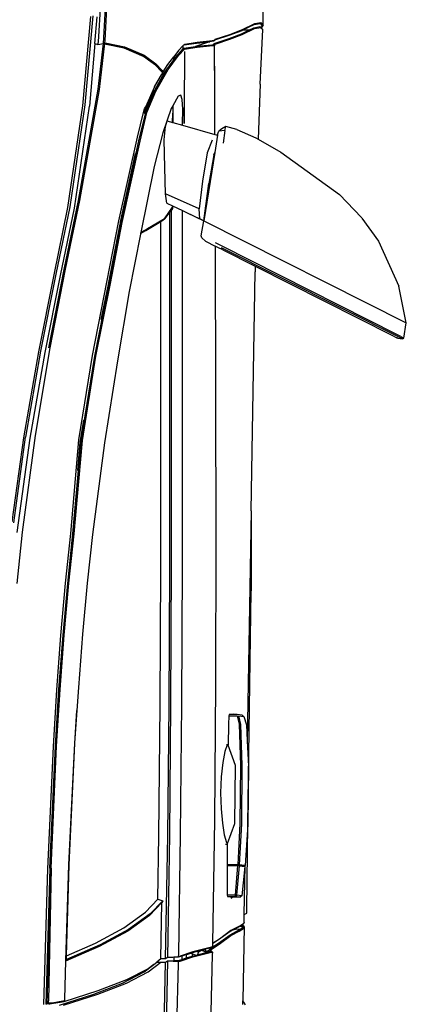
# Model space of a CAD drawing. Units: inches. Extents: x 22042254 to 25404563, y 17568978 to 17626777.
# Tile 31 of 45: x 22179875 to 22179896, y 17626279 to 17626332. Entities that reach past the tile are written whole.
import ezdxf

# ---------------------------------------------------------------- set-up
doc = ezdxf.new("R2010")
doc.units = ezdxf.units.IN
doc.header["$MEASUREMENT"] = 0
doc.layers.add('A-SITE-VEHI', color=8, linetype='Continuous', lineweight=18)
doc.layers.add('Edges', color=250, linetype='Continuous')

# ---------------------------------------------------------------- blocks, each defined once
blk = doc.blocks.new('Nissan Qashqai pl')
at = {"layer": 'Edges'}
for p, q in [((8.8918, 12.7444), (9.0186, 12.9956)), ((9.0386, 12.9907), (8.9254, 12.7664)), ((9.0186, 12.9956), (8.9731, 12.9865)), ((9.0374, 12.9925), (9.0186, 12.9956)), ((9.0356, 12.9888), (9.0333, 12.9845)), ((9.0356, 12.9888), (9.0374, 12.9925)), ((9.0386, 12.9907), (9.0374, 12.9925)), ((9.0376, 12.985), (9.0386, 12.9907)), ((8.9173, 12.961), (8.9731, 12.9865)), ((9.0333, 12.9845), (8.9232, 12.7662)), ((8.9483, 12.8082), (9.0343, 12.9785)), ((9.0343, 12.9785), (9.0347, 12.9794)), ((9.0347, 12.9794), (9.0362, 12.9822)), ((9.0362, 12.9822), (9.037, 12.9838)), ((9.0371, 12.9841), (9.037, 12.9838)), ((9.0371, 12.9841), (9.0376, 12.985)), ((9.0376, 12.985), (9.0371, 12.9847)), ((8.8885, 12.9405), (8.9173, 12.961)), ((8.8591, 12.9127), (8.8879, 12.94)), ((8.8885, 12.9405), (8.8879, 12.94)), ((8.8066, 12.84), (8.8591, 12.9127)), ((8.7908, 12.812), (8.8066, 12.84)), ((8.6489, 12.8179), (8.5719, 12.8193)), ((8.646, 12.8153), (8.6489, 12.8179)), ((8.6489, 12.8179), (8.6527, 12.8156)), ((8.6547, 12.8176), (8.6537, 12.8167)), ((8.7222, 12.8144), (8.6547, 12.8176)), ((8.646, 12.8153), (8.646, 12.8153)), ((8.6472, 12.8076), (8.646, 12.8153)), ((8.647, 12.8142), (8.6498, 12.8168)), ((8.6482, 12.8067), (8.647, 12.8142)), ((8.6546, 12.7926), (8.6472, 12.8076)), ((8.655, 12.7929), (8.6482, 12.8067)), ((8.6498, 12.8168), (8.6524, 12.8153)), ((8.651, 12.814), (8.652, 12.815)), ((8.6524, 12.8064), (8.651, 12.814)), ((8.652, 12.815), (8.6524, 12.8153)), ((8.6534, 12.8073), (8.652, 12.815)), ((8.6524, 12.8153), (8.6527, 12.8156)), ((8.655, 12.801), (8.6524, 12.8064)), ((8.6527, 12.8156), (8.6537, 12.8167)), ((8.6608, 12.7921), (8.6534, 12.8073)), ((8.6537, 12.8167), (8.6537, 12.8166)), ((8.7222, 12.8144), (8.7908, 12.812)), ((8.7785, 12.7855), (8.7891, 12.8089)), ((8.7891, 12.8089), (8.7908, 12.812)), ((8.928, 12.7679), (8.9483, 12.8082)), ((8.9483, 12.8082), (8.9552, 12.8081)), ((9.2517, 12.8031), (8.9552, 12.8081)), ((8.6606, 12.7768), (8.6546, 12.7926)), ((8.6598, 12.7913), (8.655, 12.801)), ((8.655, 12.7929), (8.655, 12.801)), ((8.6556, 12.7918), (8.655, 12.7929)), ((8.655, 12.7922), (8.655, 12.7929)), ((9.2517, 12.8031), (9.351, 12.803)), ((9.2517, 12.8031), (9.5372, 12.7983)), ((9.641, 12.7991), (9.351, 12.803)), ((9.5052, 12.7918), (9.5069, 12.7941)), ((9.5061, 12.7878), (9.5069, 12.7941)), ((9.5069, 12.7941), (9.5176, 12.7972)), ((9.5176, 12.7972), (9.5372, 12.7983)), ((9.5372, 12.7983), (9.5689, 12.7999)), ((9.5689, 12.7999), (9.641, 12.7991)), ((9.641, 12.7991), (9.6921, 12.7956)), ((9.7466, 12.7978), (9.641, 12.7991)), ((9.692, 12.7943), (9.6913, 12.7886)), ((9.6921, 12.7956), (9.692, 12.7943)), ((9.6922, 12.7943), (9.692, 12.7943)), ((9.6922, 12.7943), (9.6921, 12.7956)), ((9.7526, 12.7946), (9.6921, 12.7956)), ((9.6922, 12.7885), (9.693, 12.7955)), ((9.6922, 12.7885), (9.6922, 12.7943)), ((9.693, 12.7955), (9.7296, 12.7914)), ((9.7511, 12.7979), (9.7466, 12.7978)), ((9.7526, 12.7946), (9.7511, 12.7979)), ((9.7623, 12.7945), (9.7526, 12.7946)), ((9.7623, 12.7945), (9.7643, 12.7937)), ((9.7643, 12.7937), (9.7652, 12.7927)), ((9.7643, 12.7937), (9.7648, 12.7929)), ((9.7648, 12.7929), (9.7648, 12.7929)), ((9.7648, 12.7929), (9.7664, 12.7902)), ((9.7652, 12.7927), (9.7665, 12.7907)), ((9.7667, 12.7933), (9.7665, 12.7907)), ((9.7677, 12.7944), (9.7667, 12.7933)), ((9.7676, 12.7931), (9.7667, 12.7933)), ((9.7673, 12.7899), (9.7676, 12.7931)), ((9.769, 12.7926), (9.7676, 12.7931)), ((9.7677, 12.7944), (9.7677, 12.7944)), ((9.77, 12.7936), (9.7677, 12.7944)), ((9.7677, 12.7944), (9.8598, 12.7928)), ((9.7712, 12.7892), (9.769, 12.7926)), ((9.7734, 12.7884), (9.77, 12.7936)), ((9.8598, 12.7928), (9.8614, 12.7937)), ((9.8643, 12.7927), (9.8598, 12.7928)), ((9.8614, 12.7937), (9.8647, 12.7956)), ((8.6616, 12.7758), (8.6556, 12.7918)), ((8.6657, 12.7758), (8.6598, 12.7913)), ((8.6667, 12.7767), (8.6608, 12.7921)), ((8.7785, 12.7855), (8.7751, 12.7719)), ((9.5037, 12.7806), (9.5045, 12.7814)), ((9.5052, 12.7918), (9.5044, 12.7856)), ((9.5044, 12.7856), (9.5045, 12.7814)), ((9.5045, 12.7814), (9.5045, 12.7759)), ((9.5168, 12.7904), (9.5061, 12.7878)), ((9.5061, 12.7856), (9.5167, 12.7883)), ((9.5063, 12.7755), (9.5061, 12.7856)), ((9.5167, 12.7883), (9.5679, 12.7899)), ((9.5679, 12.792), (9.5168, 12.7904)), ((9.5678, 12.7837), (9.5426, 12.7747)), ((9.64, 12.7831), (9.5678, 12.7837)), ((9.6401, 12.7914), (9.5679, 12.792)), ((9.5679, 12.7899), (9.64, 12.7892)), ((9.64, 12.7892), (9.6912, 12.7865)), ((9.6645, 12.7737), (9.64, 12.7831)), ((9.6913, 12.7886), (9.6401, 12.7914)), ((9.6912, 12.7811), (9.6911, 12.7796)), ((9.6913, 12.7886), (9.6912, 12.7865)), ((9.6912, 12.7865), (9.6912, 12.7811)), ((9.692, 12.7811), (9.6912, 12.7811)), ((9.692, 12.7811), (9.6921, 12.7864)), ((9.692, 12.7796), (9.692, 12.7811)), ((9.6922, 12.7885), (9.6921, 12.7864)), ((9.6921, 12.7864), (9.7288, 12.7832)), ((9.7288, 12.7854), (9.6922, 12.7885)), ((9.7288, 12.7832), (9.7287, 12.7734)), ((9.7296, 12.7914), (9.7288, 12.7854)), ((9.7306, 12.7834), (9.7288, 12.7854)), ((9.7288, 12.7854), (9.7288, 12.7832)), ((9.7288, 12.7832), (9.7306, 12.7834)), ((9.7296, 12.7914), (9.7314, 12.7895)), ((9.7305, 12.7738), (9.7306, 12.7834)), ((9.7306, 12.7834), (9.7314, 12.7895)), ((9.7314, 12.7895), (9.7313, 12.7798)), ((9.7665, 12.7904), (9.7664, 12.7902)), ((9.7664, 12.7902), (9.7674, 12.7885)), ((9.7665, 12.7907), (9.7676, 12.7889)), ((9.7673, 12.7897), (9.7673, 12.7899)), ((9.7673, 12.7897), (9.7676, 12.7889)), ((9.7674, 12.7885), (9.7728, 12.7781)), ((9.7676, 12.7889), (9.7684, 12.7875)), ((9.7676, 12.7887), (9.7678, 12.7882)), ((9.7684, 12.7875), (9.7717, 12.781)), ((9.7707, 12.7848), (9.7709, 12.7893)), ((9.7717, 12.781), (9.7707, 12.7848)), ((9.7709, 12.7893), (9.7712, 12.7892)), ((9.7724, 12.7874), (9.7712, 12.7892)), ((9.7717, 12.781), (9.7738, 12.7771)), ((9.7778, 12.777), (9.7724, 12.7874)), ((9.7788, 12.778), (9.7734, 12.7884)), ((8.6667, 12.7584), (8.6606, 12.7768)), ((8.6675, 12.758), (8.6616, 12.7758)), ((8.6718, 12.7574), (8.6657, 12.7758)), ((8.6728, 12.7584), (8.6667, 12.7767)), ((8.7751, 12.7719), (8.7779, 12.7668)), ((8.7798, 12.7703), (8.7751, 12.7719)), ((8.7798, 12.7703), (8.7807, 12.763)), ((8.7798, 12.7703), (8.7954, 12.7683)), ((9.5045, 12.7759), (9.5063, 12.7755)), ((9.5063, 12.7755), (9.5168, 12.7751)), ((9.5168, 12.7751), (9.5423, 12.7746)), ((9.5423, 12.7746), (9.5422, 12.7736)), ((9.5422, 12.7736), (9.5422, 12.7725)), ((9.5422, 12.7736), (9.5424, 12.7735)), ((9.5426, 12.7747), (9.5423, 12.7746)), ((9.5426, 12.7747), (9.5424, 12.7735)), ((9.5424, 12.7735), (9.5503, 12.7706)), ((9.5503, 12.7706), (9.5641, 12.7681)), ((9.6395, 12.7676), (9.654, 12.7697)), ((9.654, 12.7697), (9.6633, 12.7726)), ((9.6633, 12.7726), (9.6645, 12.7737)), ((9.6655, 12.7733), (9.6645, 12.7737)), ((9.6655, 12.7733), (9.6911, 12.7732)), ((9.6655, 12.7713), (9.6655, 12.7733)), ((9.6911, 12.7796), (9.6911, 12.7732)), ((9.6911, 12.7732), (9.692, 12.7733)), ((9.692, 12.7733), (9.692, 12.7796)), ((9.692, 12.7733), (9.7287, 12.7734)), ((9.7287, 12.7734), (9.7305, 12.7738)), ((9.7305, 12.7738), (9.7313, 12.7798)), ((9.733, 12.7782), (9.7313, 12.7798)), ((9.7728, 12.7781), (9.7832, 12.7637)), ((9.7738, 12.7771), (9.7842, 12.7627)), ((9.7883, 12.7626), (9.7778, 12.777)), ((9.7894, 12.7636), (9.7788, 12.778)), ((8.6675, 12.758), (8.6667, 12.7584)), ((8.6679, 12.7578), (8.6675, 12.758)), ((8.6676, 12.7576), (8.6675, 12.7576)), ((8.6675, 12.7576), (8.6675, 12.7576)), ((8.6675, 12.7576), (8.6676, 12.7576)), ((8.6676, 12.7576), (8.6677, 12.7576)), ((8.6677, 12.7576), (8.6677, 12.7576)), ((8.6677, 12.7576), (8.6682, 12.7576)), ((8.6682, 12.7576), (8.6679, 12.7578)), ((8.6682, 12.7576), (8.6692, 12.7566)), ((8.6682, 12.7572), (8.6682, 12.7576)), ((8.6684, 12.7554), (8.6682, 12.7572)), ((8.6682, 12.7572), (8.6692, 12.7566)), ((8.6692, 12.7566), (8.6697, 12.7519)), ((8.6729, 12.7568), (8.6718, 12.7574)), ((8.674, 12.7578), (8.6728, 12.7584)), ((8.6733, 12.7566), (8.6729, 12.7568)), ((8.6735, 12.7544), (8.6733, 12.7566)), ((8.6742, 12.7576), (8.674, 12.7578)), ((8.6742, 12.7584), (8.6743, 12.7582)), ((8.6744, 12.755), (8.6742, 12.7576)), ((8.6744, 12.7576), (8.6742, 12.7576)), ((8.6744, 12.7578), (8.6744, 12.7576)), ((8.6773, 12.7577), (8.6744, 12.7576)), ((8.6791, 12.7578), (8.677, 12.7578)), ((8.6791, 12.7577), (8.6773, 12.7577)), ((8.7205, 12.7579), (8.6791, 12.7578)), ((8.6791, 12.7577), (8.6791, 12.7578)), ((8.6878, 12.7577), (8.6791, 12.7578)), ((8.6878, 12.7577), (8.6791, 12.7577)), ((8.6878, 12.7577), (8.6878, 12.7577)), ((8.6911, 12.7577), (8.6878, 12.7577)), ((8.7205, 12.7579), (8.6911, 12.7577)), ((8.7849, 12.7582), (8.7205, 12.7579)), ((8.7734, 12.7181), (8.7849, 12.7582)), ((8.7779, 12.7668), (8.7807, 12.763)), ((8.7849, 12.7615), (8.7807, 12.763)), ((8.7849, 12.7615), (8.7858, 12.7613)), ((8.7849, 12.7582), (8.7856, 12.7608)), ((8.7858, 12.7613), (8.7856, 12.7608)), ((8.7858, 12.7613), (8.807, 12.758)), ((8.8102, 12.7568), (8.807, 12.758)), ((8.807, 12.758), (8.8918, 12.7444)), ((8.8102, 12.7568), (8.8455, 12.7506)), ((8.9171, 12.7464), (8.9233, 12.7586)), ((8.9232, 12.7662), (8.9194, 12.7588)), ((8.925, 12.762), (8.9233, 12.7586)), ((8.9233, 12.7586), (9.2886, 12.7594)), ((8.928, 12.7679), (8.925, 12.762)), ((9.2886, 12.7594), (9.4673, 12.7589)), ((9.4673, 12.7589), (9.6358, 12.7575)), ((9.5641, 12.7681), (9.5818, 12.766)), ((9.5818, 12.766), (9.6016, 12.7651)), ((9.6016, 12.7651), (9.6215, 12.766)), ((9.6215, 12.766), (9.6395, 12.7676)), ((9.6358, 12.7575), (9.7887, 12.7552)), ((9.7832, 12.7637), (9.7887, 12.7552)), ((9.7842, 12.7627), (9.7891, 12.7552)), ((9.7933, 12.7549), (9.7883, 12.7626)), ((9.7965, 12.7526), (9.7894, 12.7636)), ((8.6684, 12.7554), (8.6685, 12.7549)), ((8.6684, 12.755), (8.6684, 12.7554)), ((8.6703, 12.7361), (8.6684, 12.755)), ((8.6697, 12.7519), (8.6698, 12.7516)), ((8.6714, 12.7353), (8.6697, 12.7519)), ((8.6698, 12.7516), (8.6755, 12.7343)), ((8.6754, 12.7353), (8.6735, 12.7544)), ((8.6764, 12.736), (8.6744, 12.755)), ((8.7917, 12.7547), (8.8075, 12.7486)), ((8.8075, 12.7486), (8.8429, 12.7426)), ((8.8918, 12.7444), (8.8455, 12.7506)), ((8.8815, 12.7228), (8.892, 12.7444)), ((8.892, 12.7444), (8.8908, 12.7421)), ((8.8911, 12.7428), (8.8919, 12.7444)), ((8.8911, 12.7428), (8.8919, 12.7444)), ((8.8919, 12.7444), (8.8911, 12.7428)), ((8.8919, 12.7444), (8.8918, 12.7444)), ((8.892, 12.7444), (8.8919, 12.7444)), ((8.8919, 12.7444), (8.8919, 12.7444)), ((8.8919, 12.7444), (8.8919, 12.7444)), ((8.9106, 12.7413), (8.892, 12.7444)), ((8.892, 12.7444), (8.892, 12.7444)), ((8.9171, 12.7464), (8.9131, 12.7421)), ((8.9171, 12.7464), (8.917, 12.7468)), ((9.7887, 12.7552), (9.7891, 12.7552)), ((9.7891, 12.7552), (9.79, 12.7552)), ((9.79, 12.7552), (9.7931, 12.7552)), ((9.7931, 12.7552), (9.7934, 12.7535)), ((9.7931, 12.7552), (9.7933, 12.7549)), ((9.7933, 12.7549), (9.7941, 12.7541)), ((9.7934, 12.7535), (9.7938, 12.7538)), ((9.7934, 12.7535), (9.7937, 12.7524)), ((9.7937, 12.7524), (9.7992, 12.7308)), ((9.7941, 12.7541), (9.7943, 12.7535)), ((9.7955, 12.7516), (9.7943, 12.7535)), ((9.7943, 12.7535), (9.7964, 12.7453)), ((9.7963, 12.7523), (9.7955, 12.7516)), ((9.7963, 12.7523), (9.7963, 12.7524)), ((9.7964, 12.7524), (9.7963, 12.7523)), ((9.7992, 12.7476), (9.7963, 12.7523)), ((9.7967, 12.7526), (9.7964, 12.7524)), ((9.7964, 12.7525), (9.7964, 12.7524)), ((9.7964, 12.7524), (9.7996, 12.7475)), ((9.7964, 12.7453), (9.7992, 12.7476)), ((9.7964, 12.7453), (9.7973, 12.7418)), ((9.7983, 12.7541), (9.7965, 12.7526)), ((9.7965, 12.7526), (9.7967, 12.7526)), ((9.7977, 12.7535), (9.7967, 12.7526)), ((9.7967, 12.7526), (9.7986, 12.7526)), ((9.7982, 12.754), (9.7977, 12.7535)), ((9.7977, 12.7444), (9.7985, 12.7451)), ((9.7985, 12.7451), (9.7977, 12.7431)), ((9.7977, 12.7431), (9.7977, 12.7444)), ((9.7983, 12.7541), (9.7982, 12.754)), ((9.7986, 12.7526), (9.7982, 12.754)), ((9.7986, 12.7544), (9.7983, 12.7541)), ((9.7989, 12.7461), (9.7985, 12.7451)), ((9.7993, 12.755), (9.7986, 12.7544)), ((9.7988, 12.7516), (9.7986, 12.7526)), ((9.7998, 12.7477), (9.7988, 12.7516)), ((9.7998, 12.7466), (9.7989, 12.7461)), ((9.7998, 12.7466), (9.7992, 12.7476)), ((9.7999, 12.7522), (9.7993, 12.755)), ((9.7993, 12.755), (9.8024, 12.7549)), ((9.7996, 12.7475), (9.7998, 12.7477)), ((9.8002, 12.7461), (9.7996, 12.7475)), ((9.8001, 12.7468), (9.7996, 12.7475)), ((9.8001, 12.7468), (9.7998, 12.7477)), ((9.8003, 12.7458), (9.7998, 12.7466)), ((9.8054, 12.7307), (9.7999, 12.7522)), ((9.8002, 12.7461), (9.8001, 12.7468)), ((9.8003, 12.7458), (9.8002, 12.7461)), ((9.8027, 12.7364), (9.8003, 12.7458)), ((9.8024, 12.7549), (9.9426, 12.7518)), ((8.6727, 12.7207), (8.6703, 12.7361)), ((8.6737, 12.7197), (8.6714, 12.7353)), ((8.6755, 12.7343), (8.6754, 12.7353)), ((8.6777, 12.7196), (8.6755, 12.7343)), ((8.6764, 12.7359), (8.6764, 12.736)), ((8.6788, 12.7205), (8.6764, 12.7359)), ((8.8429, 12.7426), (8.8771, 12.7388)), ((8.8771, 12.7388), (8.8585, 12.6969)), ((8.8895, 12.7393), (8.8771, 12.7388)), ((8.8815, 12.7228), (8.8895, 12.7393)), ((8.8908, 12.7421), (8.8895, 12.7393)), ((8.8906, 12.7418), (8.8895, 12.7393)), ((8.8906, 12.7418), (8.8911, 12.7428)), ((8.9131, 12.7421), (8.9106, 12.7413)), ((9.7977, 12.7431), (9.7973, 12.7418)), ((9.7973, 12.7418), (9.7977, 12.7409)), ((9.7973, 12.7418), (9.7977, 12.7399)), ((9.7977, 12.7399), (9.7977, 12.7409)), ((9.7977, 12.7409), (9.7987, 12.7388)), ((9.7977, 12.7399), (9.7978, 12.7397)), ((9.7987, 12.7388), (9.7978, 12.7397)), ((9.7978, 12.7397), (9.7987, 12.7362)), ((9.7987, 12.7388), (9.7992, 12.7377)), ((9.7987, 12.7362), (9.7992, 12.7377)), ((9.7987, 12.7362), (9.8002, 12.7301)), ((9.7992, 12.7377), (9.8027, 12.7364)), ((9.8014, 12.7303), (9.8031, 12.7349)), ((9.8031, 12.7349), (9.8027, 12.7364)), ((9.8043, 12.7303), (9.8031, 12.7349)), ((8.6737, 12.7197), (8.6727, 12.7207)), ((8.6746, 12.7189), (8.6737, 12.7197)), ((8.6785, 12.7189), (8.6777, 12.7196)), ((8.687, 12.7132), (8.6788, 12.7205)), ((8.6818, 12.7204), (8.7012, 12.7203)), ((8.7012, 12.7203), (8.7012, 12.7203)), ((8.7012, 12.7203), (8.7026, 12.7203)), ((8.7026, 12.7203), (8.7026, 12.7203)), ((8.7026, 12.7203), (8.7072, 12.7203)), ((8.7072, 12.7203), (8.7072, 12.7203)), ((8.7072, 12.7203), (8.7273, 12.7202)), ((8.7273, 12.7202), (8.7273, 12.7201)), ((8.7273, 12.7202), (8.7354, 12.7202)), ((8.7354, 12.7201), (8.7354, 12.7202)), ((8.7354, 12.7202), (8.742, 12.7202)), ((8.742, 12.7201), (8.742, 12.7202)), ((8.742, 12.7202), (8.742, 12.7201)), ((8.742, 12.7202), (8.742, 12.7202)), ((8.742, 12.7202), (8.7426, 12.7202)), ((8.7426, 12.7201), (8.7426, 12.7202)), ((8.7426, 12.7202), (8.7433, 12.7202)), ((8.7433, 12.7201), (8.7433, 12.7202)), ((8.7433, 12.7202), (8.7711, 12.7201)), ((8.7711, 12.7201), (8.7516, 12.72)), ((8.8793, 12.7181), (8.8815, 12.7228)), ((9.7992, 12.7308), (9.8044, 12.7151)), ((9.8002, 12.7301), (9.8008, 12.7285)), ((9.8008, 12.7285), (9.8014, 12.7303)), ((9.8008, 12.7285), (9.8014, 12.7265)), ((9.8043, 12.7303), (9.8014, 12.7303)), ((9.8014, 12.7265), (9.803, 12.723)), ((9.8014, 12.7265), (9.8026, 12.723)), ((9.803, 12.723), (9.8026, 12.723)), ((9.8026, 12.723), (9.8046, 12.7171)), ((9.8067, 12.7229), (9.803, 12.723)), ((9.8044, 12.73), (9.8043, 12.7303)), ((9.8067, 12.7229), (9.8044, 12.73)), ((9.8106, 12.715), (9.8054, 12.7307)), ((9.8086, 12.7171), (9.8067, 12.7229)), ((8.6785, 12.7189), (8.6746, 12.7189)), ((8.6805, 12.7132), (8.6746, 12.7189)), ((8.6815, 12.7162), (8.6785, 12.7189)), ((8.6805, 12.7132), (8.6884, 12.7071)), ((8.6815, 12.7162), (8.6818, 12.7154)), ((8.6817, 12.716), (8.6815, 12.7162)), ((8.6817, 12.716), (8.6818, 12.7154)), ((8.6859, 12.7122), (8.6817, 12.716)), ((8.6818, 12.7154), (8.6902, 12.7081)), ((8.6927, 12.7071), (8.6859, 12.7122)), ((8.7042, 12.7002), (8.687, 12.7132)), ((8.6917, 12.7071), (8.6884, 12.7071)), ((8.698, 12.6996), (8.6884, 12.7071)), ((8.6902, 12.7081), (8.6917, 12.7071)), ((8.6917, 12.7071), (8.7075, 12.6955)), ((8.6927, 12.7071), (8.6923, 12.7071)), ((8.7032, 12.6992), (8.6927, 12.7071)), ((8.7415, 12.7177), (8.7361, 12.7158)), ((8.7361, 12.7158), (8.7373, 12.7128)), ((8.7373, 12.7128), (8.7492, 12.7059)), ((8.7534, 12.7185), (8.7415, 12.7177)), ((8.7718, 12.7181), (8.7534, 12.7185)), ((8.7698, 12.7058), (8.7734, 12.7181)), ((8.7734, 12.7181), (8.7718, 12.7181)), ((8.8734, 12.7057), (8.8793, 12.7181)), ((9.3194, 12.7179), (8.8793, 12.7181)), ((9.4919, 12.7173), (9.3194, 12.7179)), ((9.6538, 12.7157), (9.4919, 12.7173)), ((9.802, 12.7133), (9.6538, 12.7157)), ((9.8051, 12.7132), (9.802, 12.7133)), ((9.8044, 12.7151), (9.8051, 12.7132)), ((9.8046, 12.7171), (9.8086, 12.7171)), ((9.8046, 12.7171), (9.8055, 12.7143)), ((9.8061, 12.6994), (9.8051, 12.7132)), ((9.8055, 12.7143), (9.8058, 12.7073)), ((9.8058, 12.7073), (9.8098, 12.7073)), ((9.8058, 12.7073), (9.8061, 12.6994)), ((9.8096, 12.7142), (9.8086, 12.7171)), ((9.8098, 12.7073), (9.8096, 12.7142)), ((9.8101, 12.6993), (9.8098, 12.7073)), ((9.8101, 12.6993), (9.8112, 12.7131)), ((9.8112, 12.7131), (9.8106, 12.715)), ((9.8143, 12.713), (9.8112, 12.7131)), ((9.9414, 12.71), (9.8143, 12.713)), ((8.7071, 12.6942), (8.698, 12.6996)), ((8.7302, 12.684), (8.7032, 12.6992)), ((8.7312, 12.6851), (8.7042, 12.7002)), ((8.7075, 12.6955), (8.7346, 12.6806)), ((8.7492, 12.7059), (8.7572, 12.7062)), ((8.7492, 12.7059), (8.7524, 12.704)), ((8.7524, 12.704), (8.7828, 12.6934)), ((8.7572, 12.7062), (8.7698, 12.7058)), ((8.7698, 12.7057), (8.7583, 12.706)), ((8.7678, 12.6988), (8.7698, 12.7057)), ((8.7748, 12.6967), (8.7678, 12.6988)), ((8.7698, 12.7057), (8.7698, 12.7058)), ((8.7916, 12.6954), (8.7748, 12.6967)), ((8.8259, 12.6959), (8.7916, 12.6954)), ((8.8585, 12.6969), (8.8259, 12.6959)), ((8.87, 12.6987), (8.8585, 12.6969)), ((8.87, 12.6987), (8.8734, 12.7057)), ((8.8734, 12.7057), (8.8768, 12.7057)), ((8.8751, 12.7054), (8.8768, 12.7057)), ((8.8893, 12.6956), (8.8751, 12.7054)), ((8.8768, 12.7057), (8.879, 12.704)), ((8.879, 12.704), (9.3198, 12.7039)), ((8.879, 12.704), (8.881, 12.7023)), ((9.3225, 12.7021), (8.881, 12.7023)), ((8.881, 12.7023), (8.8893, 12.6956)), ((8.8893, 12.6956), (8.9021, 12.6745)), ((8.8913, 12.6936), (8.8893, 12.6956)), ((9.3198, 12.7039), (9.4922, 12.7033)), ((9.4936, 12.7013), (9.3225, 12.7021)), ((9.4922, 12.7033), (9.654, 12.7018)), ((9.6552, 12.6997), (9.4936, 12.7013)), ((9.654, 12.7018), (9.8061, 12.6994)), ((9.8078, 12.6971), (9.6552, 12.6997)), ((9.8061, 12.6994), (9.8078, 12.6971)), ((9.8078, 12.6971), (9.8078, 12.6913)), ((9.8119, 12.697), (9.8101, 12.6993)), ((9.8101, 12.6993), (9.9411, 12.6966)), ((9.9393, 12.6944), (9.8119, 12.697)), ((9.8119, 12.6912), (9.8119, 12.697)), ((8.6864, 12.6706), (8.697, 12.685)), ((8.6875, 12.6698), (8.6979, 12.6839)), ((8.6987, 12.6845), (8.6924, 12.676)), ((8.697, 12.685), (8.7055, 12.6927)), ((8.6979, 12.6839), (8.7062, 12.6915)), ((8.7062, 12.6915), (8.6987, 12.6845)), ((8.7055, 12.6927), (8.7071, 12.6942)), ((8.7062, 12.6915), (8.7067, 12.6919)), ((8.7067, 12.6919), (8.7083, 12.6934)), ((8.7071, 12.6942), (8.7083, 12.6934)), ((8.7083, 12.6934), (8.7083, 12.6934)), ((8.7083, 12.6934), (8.7083, 12.6934)), ((8.7102, 12.6923), (8.7083, 12.6934)), ((8.7083, 12.6934), (8.7083, 12.6934)), ((8.7108, 12.6919), (8.7102, 12.6923)), ((8.7102, 12.6923), (8.7102, 12.6923)), ((8.7257, 12.6833), (8.7108, 12.6919)), ((8.7248, 12.6836), (8.7108, 12.6919)), ((8.7257, 12.6833), (8.7248, 12.6836)), ((8.7257, 12.6832), (8.7257, 12.6833)), ((8.7257, 12.6832), (8.7508, 12.672)), ((8.7529, 12.6741), (8.7302, 12.684)), ((8.7574, 12.6737), (8.7312, 12.6851)), ((8.7828, 12.6934), (8.8245, 12.6828)), ((8.8245, 12.6828), (8.9063, 12.6663)), ((8.8927, 12.6913), (8.8913, 12.6936)), ((9.3224, 12.6911), (8.8927, 12.6913)), ((8.9041, 12.6725), (8.8927, 12.6913)), ((9.3225, 12.6911), (9.3224, 12.6911)), ((9.4936, 12.6904), (9.3225, 12.6911)), ((9.6552, 12.6888), (9.4936, 12.6904)), ((9.7337, 12.6875), (9.6552, 12.6888)), ((9.7337, 12.6875), (9.7357, 12.6935)), ((9.7499, 12.6721), (9.7337, 12.6875)), ((9.7357, 12.6935), (9.7378, 12.6924)), ((9.7357, 12.6935), (9.7519, 12.678)), ((9.7378, 12.6924), (9.754, 12.677)), ((9.8078, 12.6913), (9.7378, 12.6924)), ((9.8078, 12.6913), (9.8119, 12.6862)), ((9.8241, 12.6756), (9.8119, 12.6912)), ((9.8119, 12.6862), (9.8119, 12.6912)), ((9.8147, 12.6826), (9.8119, 12.6862)), ((8.6759, 12.6459), (8.6864, 12.6706)), ((8.6883, 12.6704), (8.6777, 12.6457)), ((8.6924, 12.676), (8.6883, 12.6704)), ((8.6924, 12.676), (8.6924, 12.6762)), ((8.7346, 12.6806), (8.7491, 12.6738)), ((8.7346, 12.6806), (8.7577, 12.6709)), ((8.7508, 12.672), (8.7491, 12.6738)), ((8.7491, 12.6738), (8.7576, 12.6699)), ((8.7532, 12.6708), (8.7508, 12.672)), ((8.7529, 12.6741), (8.7577, 12.6709)), ((8.757, 12.6724), (8.7529, 12.6741)), ((8.7575, 12.6698), (8.7532, 12.6708)), ((8.7587, 12.672), (8.757, 12.6724)), ((8.7931, 12.6653), (8.7574, 12.6737)), ((8.7582, 12.6707), (8.7576, 12.6699)), ((8.7577, 12.6709), (8.7582, 12.6707)), ((8.759, 12.6717), (8.7582, 12.6707)), ((8.7587, 12.672), (8.759, 12.6717)), ((8.7591, 12.6719), (8.7587, 12.672)), ((8.7591, 12.6719), (8.759, 12.6717)), ((8.7925, 12.664), (8.7591, 12.6719)), ((8.9021, 12.6745), (8.9063, 12.6663)), ((8.9075, 12.6661), (8.9041, 12.6725)), ((9.7692, 12.6453), (9.7499, 12.6721)), ((9.7519, 12.678), (9.7713, 12.6512)), ((9.754, 12.677), (9.7733, 12.6502)), ((9.8147, 12.6826), (9.8147, 12.6826)), ((9.8147, 12.6826), (9.8201, 12.6756)), ((9.8241, 12.6706), (9.8147, 12.6826)), ((9.8201, 12.6756), (9.8338, 12.6486)), ((9.8378, 12.6485), (9.8241, 12.6756)), ((9.8378, 12.6435), (9.8241, 12.6706)), ((8.6772, 12.6454), (8.6875, 12.6698)), ((8.7576, 12.6699), (8.7575, 12.6698)), ((8.7881, 12.6621), (8.7575, 12.6698)), ((8.8918, 12.6392), (8.7881, 12.6621)), ((8.8941, 12.6418), (8.7925, 12.664)), ((8.8942, 12.6432), (8.7931, 12.6653)), ((8.8083, 12.6591), (8.8954, 12.6403)), ((8.9063, 12.6663), (8.9075, 12.6661)), ((8.9075, 12.6661), (8.9087, 12.6658)), ((8.9087, 12.6658), (8.9797, 12.6518)), ((8.9797, 12.6518), (9.0656, 12.6372)), ((9.7713, 12.6512), (9.7905, 12.6158)), ((9.7733, 12.6502), (9.7925, 12.6148)), ((9.8338, 12.6486), (9.8475, 12.613)), ((9.8516, 12.6129), (9.8378, 12.6485)), ((8.6716, 12.6242), (8.6759, 12.6459)), ((8.6772, 12.6454), (8.6721, 12.6201)), ((8.6777, 12.6457), (8.6727, 12.6213)), ((8.9679, 12.6241), (8.8918, 12.6392)), ((9.0601, 12.6092), (8.8941, 12.6418)), ((8.9696, 12.6285), (8.8942, 12.6432)), ((8.8961, 12.6401), (8.9704, 12.6257)), ((9.0656, 12.6372), (9.1676, 12.6212)), ((9.7885, 12.6099), (9.7692, 12.6453)), ((9.8516, 12.6079), (9.8378, 12.6435)), ((8.6197, 12.6241), (8.6683, 12.6215)), ((8.6721, 12.6201), (8.6204, 12.6229)), ((8.6683, 12.6215), (8.671, 12.6214)), ((8.671, 12.6214), (8.6716, 12.6242)), ((9.0591, 12.6065), (8.9679, 12.6241)), ((9.06, 12.6106), (8.9696, 12.6285)), ((8.9704, 12.6257), (8.9708, 12.6256)), ((8.9708, 12.6256), (9.0143, 12.6169)), ((8.622, 12.6161), (8.6699, 12.6132)), ((8.6721, 12.6093), (8.6387, 12.6123)), ((8.6699, 12.6132), (8.6721, 12.613)), ((8.671, 12.6214), (8.6721, 12.6201)), ((8.6727, 12.6213), (8.6721, 12.6201)), ((8.6733, 12.6129), (8.6721, 12.6201)), ((8.7287, 12.6134), (8.6721, 12.6201)), ((8.6721, 12.6127), (8.6721, 12.613)), ((8.6721, 12.613), (8.6733, 12.6129)), ((8.6721, 12.6093), (8.6733, 12.6129)), ((8.6721, 12.6093), (8.7496, 12.6025)), ((8.6727, 12.6213), (8.6753, 12.621)), ((8.6753, 12.621), (8.7292, 12.6146)), ((8.8666, 12.5888), (8.7287, 12.6134)), ((8.7292, 12.6146), (8.8666, 12.5901)), ((9.1644, 12.5938), (9.06, 12.6106)), ((9.1676, 12.6212), (9.2814, 12.6065)), ((9.8039, 12.5741), (9.7885, 12.6099)), ((9.7905, 12.6158), (9.8087, 12.574)), ((9.7925, 12.6148), (9.8107, 12.573)), ((9.8475, 12.613), (9.8611, 12.5708)), ((9.8652, 12.5704), (9.8516, 12.6129)), ((8.6375, 12.6066), (8.7481, 12.5968)), ((8.6386, 12.6037), (8.7491, 12.594)), ((8.8761, 12.5839), (8.7496, 12.6025)), ((9.1639, 12.5895), (9.0591, 12.6065)), ((9.1645, 12.5924), (9.0601, 12.6092)), ((9.2814, 12.6065), (9.3416, 12.5999)), ((9.3416, 12.5999), (9.4048, 12.5941)), ((9.8652, 12.5654), (9.8516, 12.6079)), ((8.7481, 12.5968), (8.8745, 12.5782)), ((8.7491, 12.594), (8.8754, 12.5755)), ((8.8666, 12.5901), (8.9521, 12.5726)), ((8.9522, 12.5713), (8.8666, 12.5888)), ((9.1393, 12.5951), (9.1647, 12.591)), ((9.2801, 12.5794), (9.1639, 12.5895)), ((9.2803, 12.5836), (9.1644, 12.5938)), ((9.2804, 12.5821), (9.1645, 12.5924)), ((9.1647, 12.591), (9.1668, 12.5908)), ((9.1668, 12.5908), (9.2019, 12.5877)), ((9.4048, 12.5941), (9.471, 12.5888)), ((9.471, 12.5888), (9.4997, 12.5869)), ((9.5404, 12.5844), (9.4997, 12.5869)), ((9.4997, 12.5869), (9.5403, 12.5842)), ((8.8745, 12.5782), (8.9583, 12.5609)), ((8.8754, 12.5755), (8.9591, 12.5583)), ((8.9598, 12.5666), (8.8761, 12.5839)), ((9.3418, 12.5729), (9.2801, 12.5794)), ((9.3418, 12.5771), (9.2803, 12.5836)), ((9.3419, 12.5756), (9.2804, 12.5821)), ((9.4062, 12.5713), (9.3418, 12.5771)), ((9.4064, 12.5671), (9.3418, 12.5729)), ((9.4063, 12.5699), (9.3419, 12.5756)), ((9.5403, 12.5842), (9.6913, 12.5767)), ((9.6912, 12.5774), (9.5404, 12.5844)), ((9.8039, 12.5741), (9.6912, 12.5774)), ((9.6913, 12.5767), (9.8099, 12.573)), ((9.8087, 12.574), (9.8039, 12.5741)), ((9.8099, 12.573), (9.8087, 12.574)), ((9.8099, 12.573), (9.8107, 12.573)), ((9.8107, 12.573), (9.8573, 12.5716)), ((8.9521, 12.5726), (9.0495, 12.5536)), ((9.0497, 12.5523), (8.9522, 12.5713)), ((8.9583, 12.5609), (9.0538, 12.5419)), ((9.0552, 12.5477), (8.9598, 12.5666)), ((9.4735, 12.5663), (9.4062, 12.5713)), ((9.4736, 12.5648), (9.4063, 12.5699)), ((9.4739, 12.5621), (9.4064, 12.5671)), ((9.5437, 12.5619), (9.4735, 12.5663)), ((9.5438, 12.5605), (9.4736, 12.5648)), ((9.5443, 12.5579), (9.4739, 12.5621)), ((9.6953, 12.5549), (9.5437, 12.5619)), ((9.6954, 12.5535), (9.5438, 12.5605)), ((9.8573, 12.5716), (9.8603, 12.5715)), ((9.8603, 12.5715), (9.8605, 12.5696)), ((9.8611, 12.5708), (9.8603, 12.5715)), ((9.8605, 12.5696), (9.8626, 12.5564)), ((9.8612, 12.5707), (9.8611, 12.5708)), ((9.8612, 12.5707), (9.8615, 12.5688)), ((9.8615, 12.5688), (9.8635, 12.5556)), ((8.9591, 12.5583), (9.0546, 12.5394)), ((9.0495, 12.5536), (9.1584, 12.5351)), ((9.696, 12.551), (9.5443, 12.5579)), ((9.6953, 12.5549), (9.8598, 12.5517)), ((9.6953, 12.5549), (9.863, 12.5497)), ((9.6954, 12.5535), (9.8641, 12.5483)), ((9.8644, 12.5459), (9.696, 12.551)), ((9.8629, 12.5516), (9.8598, 12.5517)), ((9.8626, 12.5564), (9.8627, 12.5532)), ((9.8637, 12.5532), (9.8627, 12.5532)), ((9.8627, 12.5532), (9.8629, 12.5516)), ((9.8629, 12.5516), (9.863, 12.5497)), ((9.8641, 12.5483), (9.863, 12.5497)), ((9.8635, 12.5556), (9.8637, 12.5532)), ((9.8643, 12.5532), (9.8637, 12.5532)), ((9.8637, 12.5532), (9.8638, 12.5508)), ((9.8638, 12.5508), (9.8641, 12.5483)), ((9.0538, 12.5419), (9.1605, 12.5233)), ((9.0546, 12.5394), (9.1612, 12.5208)), ((9.1617, 12.5292), (9.0552, 12.5477)), ((9.1584, 12.5351), (9.2783, 12.5191)), ((9.2789, 12.5131), (9.1617, 12.5292)), ((9.2669, 12.5088), (9.1605, 12.5233)), ((9.1612, 12.5208), (9.2656, 12.5065)), ((9.2783, 12.5191), (9.3422, 12.5126))]:
    blk.add_line(p, q, dxfattribs=at)
blk = doc.blocks.new('CAR')
blk.add_blockref('Nissan Qashqai pl', (-9.7433, -11.9151))

msp = doc.modelspace()

# ---------------------------------------------------------------- block references
at = {"layer": 'A-SITE-VEHI', "xscale": 43.56002006885659, "yscale": 43.56002006885659, "zscale": 43.56002006885659, "rotation": 270}
msp.add_blockref('CAR', (22179848.861, 17626284.325), dxfattribs=at)

doc.saveas('drawing.dxf')
